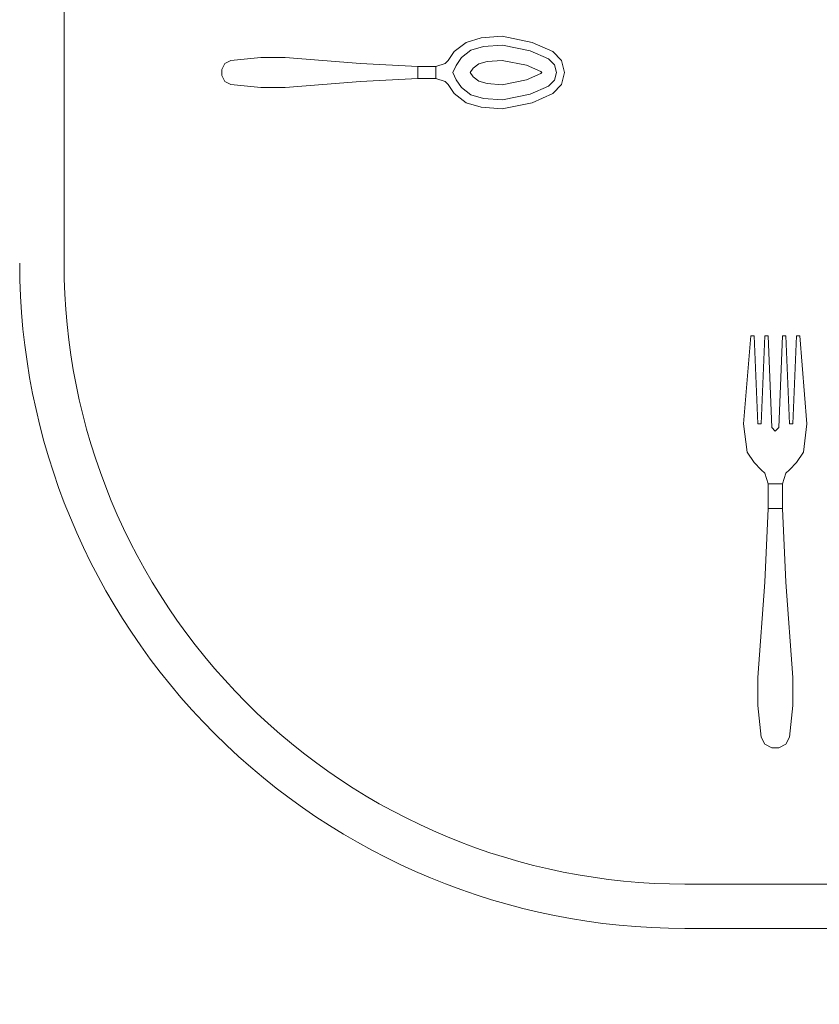
# Model space of a CAD drawing. Units: inches. Extents: x 375 to 1122, y 27 to 1069.
# Tile 9 of 155: x 705.14 to 719.12, y 253.38 to 270.59. Entities that reach past the tile are written whole.
import ezdxf

# ---------------------------------------------------------------- set-up
doc = ezdxf.new("R2010")
doc.units = ezdxf.units.IN
doc.layers.add('A-ANNO-DIMS', color=2, linetype='Continuous', lineweight=18)
doc.layers.add('Furniture', color=30, linetype='Continuous', lineweight=18)
doc.styles.get("Standard").update_dxf_attribs({"font": 'arial.ttf'})
doc.dimstyles.new('ISO-25', dxfattribs={"dimtxt": 12, "dimasz": 2.5, "dimexe": 1.5, "dimexo": 1.5, "dimtad": 1, "dimdec": 1, "dimlunit": 3, "dimtxsty": 'Standard', "dimblk": 'ARCHTICK', "dimcen": 2.5, "dimadec": 0, "dimazin": 0, "dimtfac": 1, "dimtdec": 1, "dimtmove": 0, "dimatfit": 3, "dimfxl": 1.5, "dimfxlon": 1, "dimarcsym": 0})

# ---------------------------------------------------------------- blocks, each defined once
blk = doc.blocks.new('A$C403C54AD')
for p, q in [((2.27071, 1.26108, -0.0006), (2.27071, 0.79569, -0.0006)), ((2.2901, 1.26108, -0.0006), (2.2901, 0.79569, -0.0006)), ((2.08179, 0.82287, -0.05014), (2.08641, 0.82595, -0.04968)), ((2.08179, 0.82287, -0.05322), (2.08641, 0.82595, -0.05276)), ((0.83575, 0.52421, -0.0006), (1.99923, 0.52421, -0.0006))]:
    blk.add_line(p, q)
for radius in [0.27148, 0.29087]:
    blk.add_arc((1.99923, 0.79569, -0.0006), radius, 270, 0)
for points, invisible_edges in [([(2.06948, 0.84288, -0.04954), (2.06948, 0.84903, -0.04954), (2.031, 0.84596, -0.04244), (2.031, 0.84442, -0.04244)], 1), ([(2.06948, 0.84288, -0.05262), (2.06948, 0.84903, -0.05262), (2.031, 0.84596, -0.04552), (2.031, 0.84442, -0.04552)], 1), ([(2.08179, 0.84749, -0.05014), (2.06948, 0.84134, -0.04954), (2.06948, 0.84288, -0.04954), (2.06948, 0.84903, -0.04954)], 5), ([(2.08179, 0.84749, -0.05322), (2.06948, 0.84134, -0.05262), (2.06948, 0.84288, -0.05262), (2.06948, 0.84903, -0.05262)], 5), ([(2.08179, 0.84749, -0.05014), (2.08179, 0.84749, -0.05322), (2.06948, 0.84903, -0.05262), (2.06948, 0.84903, -0.04954)], 1), ([(2.08179, 0.84749, -0.05014), (2.07268, 0.83518, -0.04994), (2.07102, 0.83672, -0.04979), (2.06948, 0.84134, -0.04954)], 13), ([(2.08179, 0.84749, -0.05322), (2.07268, 0.83518, -0.05301), (2.07102, 0.83672, -0.05286), (2.06948, 0.84134, -0.05262)], 13), ([(2.08179, 0.84749, -0.05014), (2.07268, 0.83518, -0.04994), (2.08179, 0.82287, -0.05014), (2.08179, 0.84749, -0.05014)], 7), ([(2.08179, 0.84749, -0.05322), (2.07268, 0.83518, -0.05301), (2.08179, 0.82287, -0.05322), (2.08179, 0.84749, -0.05322)], 7), ([(2.08641, 0.84442, -0.04968), (2.08641, 0.82595, -0.04968), (2.08179, 0.82287, -0.05014), (2.08179, 0.84749, -0.05014)], 5), ([(2.08641, 0.84442, -0.05276), (2.08641, 0.82595, -0.05276), (2.08179, 0.82287, -0.05322), (2.08179, 0.84749, -0.05322)], 5), ([(2.08641, 0.84442, -0.05276), (2.08641, 0.84442, -0.04968), (2.08179, 0.84749, -0.05014), (2.08179, 0.84749, -0.05322)], 4), ([(2.08949, 0.82902, -0.05152), (2.08949, 0.84134, -0.05152), (2.08641, 0.84442, -0.05276), (2.08641, 0.82595, -0.05276)], 5), ([(2.08949, 0.82902, -0.04844), (2.08949, 0.84134, -0.04844), (2.08641, 0.84442, -0.04968), (2.08641, 0.82595, -0.04968)], 5), ([(2.06948, 0.84134, -0.04954), (2.07102, 0.83672, -0.04979), (2.031, 0.83826, -0.04244), (2.031, 0.8398, -0.04244)], 1), ([(2.06948, 0.84134, -0.05262), (2.07102, 0.83672, -0.05286), (2.031, 0.83826, -0.04552), (2.031, 0.8398, -0.04552)], 1), ([(2.09103, 0.83056, -0.04739), (2.09103, 0.8398, -0.04739), (2.08949, 0.84134, -0.04844), (2.08949, 0.82902, -0.04844)], 5), ([(2.09103, 0.83056, -0.05018), (2.09103, 0.8398, -0.05018), (2.08949, 0.84134, -0.05152), (2.08949, 0.82902, -0.05152)], 5), ([(2.09103, 0.8398, -0.05018), (2.09103, 0.8398, -0.04739), (2.08949, 0.84134, -0.04844), (2.08949, 0.84134, -0.05152)], 1), ([(2.09564, 0.83826, -0.04504), (2.09564, 0.8321, -0.04504), (2.09103, 0.83056, -0.04739), (2.09103, 0.8398, -0.04739)], 4), ([(2.09564, 0.83826, -0.04763), (2.09564, 0.8321, -0.04763), (2.09103, 0.83056, -0.05018), (2.09103, 0.8398, -0.05018)], 4), ([(2.09564, 0.83826, -0.04504), (2.09564, 0.83826, -0.04763), (2.09103, 0.8398, -0.05018), (2.09103, 0.8398, -0.04739)], 5), ([(2.13874, 0.8398, -0.04587), (2.13874, 0.83056, -0.04587), (2.10642, 0.8321, -0.04296), (2.10642, 0.83826, -0.04296)], 1), ([(2.13874, 0.8398, -0.04587), (2.13874, 0.8398, -0.04895), (2.10642, 0.83826, -0.04555), (2.10642, 0.83826, -0.04296)], 5), ([(2.13874, 0.8398, -0.04895), (2.13874, 0.83056, -0.04895), (2.10642, 0.8321, -0.04555), (2.10642, 0.83826, -0.04555)], 1), ([(2.1803, 0.82749, -0.04825), (2.1803, 0.84288, -0.04825), (2.13874, 0.8398, -0.04587), (2.13874, 0.83056, -0.04587)], 5), ([(2.1803, 0.82749, -0.05289), (2.1803, 0.84288, -0.05289), (2.13874, 0.8398, -0.04895), (2.13874, 0.83056, -0.04895)], 5), ([(2.1803, 0.84288, -0.05289), (2.1803, 0.84288, -0.04825), (2.13874, 0.8398, -0.04587), (2.13874, 0.8398, -0.04895)], 4), ([(2.19261, 0.84288, -0.04858), (2.19261, 0.82749, -0.04858), (2.1803, 0.82749, -0.04825), (2.1803, 0.84288, -0.04825)], 5), ([(2.19261, 0.84288, -0.05321), (2.19261, 0.82749, -0.05321), (2.1803, 0.82749, -0.05289), (2.1803, 0.84288, -0.05289)], 5), ([(2.20647, 0.82902, -0.04855), (2.20647, 0.84134, -0.04855), (2.19261, 0.84288, -0.04858), (2.19261, 0.82749, -0.04858)], 5), ([(2.20647, 0.82902, -0.05318), (2.20647, 0.84134, -0.05318), (2.19261, 0.84288, -0.05321), (2.19261, 0.82749, -0.05321)], 5), ([(2.20954, 0.8398, -0.0483), (2.20954, 0.83056, -0.0483), (2.20647, 0.82902, -0.04855), (2.20647, 0.84134, -0.04855)], 5), ([(2.20954, 0.8398, -0.05294), (2.20954, 0.83056, -0.05294), (2.20647, 0.82902, -0.05318), (2.20647, 0.84134, -0.05318)], 5), ([(2.21108, 0.83364, -0.04847), (2.21108, 0.83672, -0.04847), (2.20954, 0.8398, -0.0483), (2.20954, 0.83056, -0.0483)], 4), ([(2.21108, 0.83364, -0.0526), (2.21108, 0.83672, -0.0526), (2.20954, 0.8398, -0.05294), (2.20954, 0.83056, -0.05294)], 4), ([(2.10642, 0.83826, -0.04555), (2.10642, 0.83826, -0.04296), (2.09564, 0.83826, -0.04504), (2.09564, 0.83826, -0.04763)], 5), ([(2.07102, 0.83364, -0.04979), (2.06948, 0.82902, -0.04954), (2.031, 0.83056, -0.04244), (2.031, 0.8321, -0.04244)], 1), ([(2.07102, 0.83364, -0.05286), (2.06948, 0.82902, -0.05262), (2.031, 0.83056, -0.04552), (2.031, 0.8321, -0.04552)], 1), ([(2.08179, 0.82287, -0.05014), (2.07268, 0.83518, -0.04994), (2.07102, 0.83364, -0.04979), (2.06948, 0.82902, -0.04954)], 13), ([(2.08179, 0.82287, -0.05322), (2.07268, 0.83518, -0.05301), (2.07102, 0.83364, -0.05286), (2.06948, 0.82902, -0.05262)], 13), ([(2.09564, 0.8321, -0.04763), (2.09564, 0.8321, -0.04504), (2.09103, 0.83056, -0.04739), (2.09103, 0.83056, -0.05018)], 5), ([(2.09564, 0.8321, -0.04763), (2.09564, 0.8321, -0.04504), (2.10642, 0.8321, -0.04296), (2.10642, 0.8321, -0.04555)], 5), ([(2.10642, 0.8321, -0.04296), (2.10642, 0.8321, -0.04555), (2.13874, 0.83056, -0.04895), (2.13874, 0.83056, -0.04587)], 5), ([(2.06948, 0.82749, -0.04954), (2.06948, 0.82133, -0.04954), (2.031, 0.82441, -0.04244), (2.031, 0.82595, -0.04244)], 1), ([(2.06948, 0.82749, -0.05262), (2.06948, 0.82133, -0.05262), (2.031, 0.82441, -0.04552), (2.031, 0.82595, -0.04552)], 1), ([(2.08179, 0.82287, -0.05014), (2.06948, 0.82902, -0.04954), (2.06948, 0.82749, -0.04954), (2.06948, 0.82133, -0.04954)], 5), ([(2.08179, 0.82287, -0.05322), (2.06948, 0.82902, -0.05262), (2.06948, 0.82749, -0.05262), (2.06948, 0.82133, -0.05262)], 5), ([(2.09103, 0.83056, -0.04739), (2.09103, 0.83056, -0.05018), (2.08949, 0.82902, -0.05152), (2.08949, 0.82902, -0.04844)], 1), ([(2.13874, 0.83056, -0.04895), (2.13874, 0.83056, -0.04587), (2.1803, 0.82749, -0.04825), (2.1803, 0.82749, -0.05289)], 1), ([(2.08179, 0.82287, -0.05322), (2.08179, 0.82287, -0.05014), (2.06948, 0.82133, -0.04954), (2.06948, 0.82133, -0.05262)], 1), ([(2.08641, 0.82595, -0.04968), (2.08641, 0.82595, -0.05276), (2.08179, 0.82287, -0.05322), (2.08179, 0.82287, -0.05014)], 4), ([(1.90985, 0.73605, -0.02421), (1.9066, 0.73789, -0.02157), (1.91055, 0.74173, -0.02048), (1.91253, 0.73867, -0.02365)], 5), ([(1.90985, 0.73605, -0.02289), (1.9066, 0.73789, -0.02025), (1.91055, 0.74173, -0.01916), (1.91253, 0.73867, -0.02233)], 5), ([(1.91055, 0.74173, -0.02048), (1.91253, 0.73867, -0.02365), (1.91583, 0.73948, -0.02346), (1.91583, 0.74304, -0.02029)], 5), ([(1.91055, 0.74173, -0.01916), (1.91253, 0.73867, -0.02233), (1.91583, 0.73948, -0.02215), (1.91583, 0.74304, -0.01897)], 5), ([(1.92111, 0.74173, -0.02048), (1.91914, 0.73867, -0.02365), (1.91583, 0.73948, -0.02346), (1.91583, 0.74304, -0.02029)], 5), ([(1.92111, 0.74173, -0.01916), (1.91914, 0.73867, -0.02233), (1.91583, 0.73948, -0.02215), (1.91583, 0.74304, -0.01897)], 5), ([(1.92182, 0.73605, -0.02421), (1.92507, 0.73789, -0.02157), (1.92111, 0.74173, -0.02048), (1.91914, 0.73867, -0.02365)], 5), ([(1.92182, 0.73605, -0.02289), (1.92507, 0.73789, -0.02025), (1.92111, 0.74173, -0.01916), (1.91914, 0.73867, -0.02233)], 5), ([(1.90264, 0.72882, -0.0234), (1.90634, 0.72802, -0.02592), (1.90985, 0.73605, -0.02421), (1.9066, 0.73789, -0.02157)], 5), ([(1.90264, 0.72882, -0.02208), (1.90634, 0.72802, -0.0246), (1.90985, 0.73605, -0.02289), (1.9066, 0.73789, -0.02025)], 5), ([(1.9154, 0.73267, -0.02578), (1.91253, 0.73867, -0.02233), (1.90985, 0.73605, -0.02289), (1.9154, 0.73267, -0.02578)], 5), ([(1.9154, 0.73267, -0.0271), (1.91253, 0.73867, -0.02365), (1.90985, 0.73605, -0.02421), (1.9154, 0.73267, -0.0271)], 5), ([(1.91583, 0.73948, -0.02215), (1.91583, 0.73309, -0.02564), (1.9154, 0.73267, -0.02578), (1.91253, 0.73867, -0.02233)], 5), ([(1.91583, 0.73948, -0.02346), (1.91583, 0.73309, -0.02696), (1.9154, 0.73267, -0.0271), (1.91253, 0.73867, -0.02365)], 5), ([(1.91583, 0.73948, -0.02215), (1.91583, 0.73309, -0.02564), (1.91627, 0.73267, -0.02578), (1.91914, 0.73867, -0.02233)], 5), ([(1.91583, 0.73948, -0.02346), (1.91583, 0.73309, -0.02696), (1.91627, 0.73267, -0.0271), (1.91914, 0.73867, -0.02365)], 5), ([(1.91627, 0.73267, -0.02578), (1.91914, 0.73867, -0.02233), (1.92182, 0.73605, -0.02289), (1.91627, 0.73267, -0.02578)], 5), ([(1.91627, 0.73267, -0.0271), (1.91914, 0.73867, -0.02365), (1.92182, 0.73605, -0.02421), (1.91627, 0.73267, -0.0271)], 5), ([(1.92903, 0.72882, -0.0234), (1.92532, 0.72802, -0.02592), (1.92182, 0.73605, -0.02421), (1.92507, 0.73789, -0.02157)], 5), ([(1.92903, 0.72882, -0.02208), (1.92532, 0.72802, -0.0246), (1.92182, 0.73605, -0.02289), (1.92507, 0.73789, -0.02025)], 5), ([(1.90985, 0.73605, -0.02421), (1.9154, 0.73267, -0.0271), (1.91266, 0.72644, -0.02873), (1.90634, 0.72802, -0.02592)], 5), ([(1.90985, 0.73605, -0.02289), (1.9154, 0.73267, -0.02578), (1.91266, 0.72644, -0.02741), (1.90634, 0.72802, -0.0246)], 5), ([(1.9154, 0.73267, -0.0271), (1.91627, 0.73267, -0.0271), (1.91901, 0.72644, -0.02873), (1.91266, 0.72644, -0.02873)], 5), ([(1.9154, 0.73267, -0.02578), (1.91627, 0.73267, -0.02578), (1.91901, 0.72644, -0.02741), (1.91266, 0.72644, -0.02741)], 5), ([(1.91583, 0.73309, -0.02564), (1.91627, 0.73267, -0.02578), (1.9154, 0.73267, -0.02578), (1.91583, 0.73309, -0.02564)], 2), ([(1.91583, 0.73309, -0.02696), (1.91627, 0.73267, -0.0271), (1.9154, 0.73267, -0.0271), (1.91583, 0.73309, -0.02696)], 2), ([(1.92182, 0.73605, -0.02421), (1.91627, 0.73267, -0.0271), (1.91901, 0.72644, -0.02873), (1.92532, 0.72802, -0.02592)], 5), ([(1.92182, 0.73605, -0.02289), (1.91627, 0.73267, -0.02578), (1.91901, 0.72644, -0.02741), (1.92532, 0.72802, -0.0246)], 5), ([(1.90388, 0.71589, -0.0279), (1.9, 0.71579, -0.02544), (1.90264, 0.72882, -0.0234), (1.90634, 0.72802, -0.02592)], 5), ([(1.90388, 0.71589, -0.02658), (1.9, 0.71579, -0.02412), (1.90264, 0.72882, -0.02208), (1.90634, 0.72802, -0.0246)], 5), ([(1.91266, 0.72644, -0.02741), (1.90634, 0.72802, -0.0246), (1.90388, 0.71589, -0.02658), (1.91051, 0.71583, -0.02912)], 5), ([(1.91266, 0.72644, -0.02873), (1.90634, 0.72802, -0.02592), (1.90388, 0.71589, -0.0279), (1.91051, 0.71583, -0.03044)], 5), ([(1.91901, 0.72644, -0.02741), (1.92532, 0.72802, -0.0246), (1.92778, 0.71589, -0.02658), (1.92116, 0.71583, -0.02912)], 5), ([(1.91901, 0.72644, -0.02873), (1.92532, 0.72802, -0.02592), (1.92778, 0.71589, -0.0279), (1.92116, 0.71583, -0.03044)], 5), ([(1.92778, 0.71589, -0.0279), (1.93166, 0.71579, -0.02544), (1.92903, 0.72882, -0.0234), (1.92532, 0.72802, -0.02592)], 5), ([(1.92778, 0.71589, -0.02658), (1.93166, 0.71579, -0.02412), (1.92903, 0.72882, -0.02208), (1.92532, 0.72802, -0.0246)], 5), ([(1.91901, 0.72644, -0.02741), (1.91266, 0.72644, -0.02741), (1.91051, 0.71583, -0.02912), (1.92116, 0.71583, -0.02912)], 5), ([(1.91901, 0.72644, -0.02873), (1.91266, 0.72644, -0.02873), (1.91051, 0.71583, -0.03044), (1.92116, 0.71583, -0.03044)], 5), ([(1.90066, 0.70658, -0.02499), (1.90447, 0.70765, -0.02747), (1.90388, 0.71589, -0.02658), (1.9, 0.71579, -0.02412)], 5), ([(1.90066, 0.70658, -0.02631), (1.90447, 0.70765, -0.02879), (1.90388, 0.71589, -0.0279), (1.9, 0.71579, -0.02544)], 5), ([(1.90388, 0.71589, -0.0279), (1.91051, 0.71583, -0.03044), (1.91098, 0.70922, -0.03139), (1.90447, 0.70765, -0.02879)], 5), ([(1.90388, 0.71589, -0.02658), (1.91051, 0.71583, -0.02912), (1.91098, 0.70922, -0.03007), (1.90447, 0.70765, -0.02747)], 5), ([(1.91051, 0.71583, -0.03044), (1.92116, 0.71583, -0.03044), (1.92068, 0.70922, -0.03139), (1.91098, 0.70922, -0.03139)], 5), ([(1.91051, 0.71583, -0.02912), (1.92116, 0.71583, -0.02912), (1.92068, 0.70922, -0.03007), (1.91098, 0.70922, -0.03007)], 5), ([(1.92778, 0.71589, -0.0279), (1.92116, 0.71583, -0.03044), (1.92068, 0.70922, -0.03139), (1.92719, 0.70765, -0.02879)], 5), ([(1.92778, 0.71589, -0.02658), (1.92116, 0.71583, -0.02912), (1.92068, 0.70922, -0.03007), (1.92719, 0.70765, -0.02747)], 5), ([(1.931, 0.70658, -0.02499), (1.92719, 0.70765, -0.02747), (1.92778, 0.71589, -0.02658), (1.93166, 0.71579, -0.02412)], 5), ([(1.931, 0.70658, -0.02631), (1.92719, 0.70765, -0.02879), (1.92778, 0.71589, -0.0279), (1.93166, 0.71579, -0.02544)], 5), ([(1.90613, 0.70213, -0.02798), (1.90264, 0.69998, -0.02539), (1.90066, 0.70658, -0.02499), (1.90447, 0.70765, -0.02747)], 5), ([(1.90613, 0.70213, -0.0293), (1.90264, 0.69998, -0.02671), (1.90066, 0.70658, -0.02631), (1.90447, 0.70765, -0.02879)], 5), ([(1.91098, 0.70922, -0.03007), (1.90447, 0.70765, -0.02747), (1.90613, 0.70213, -0.02798), (1.9121, 0.7055, -0.0303)], 5), ([(1.92068, 0.70922, -0.03139), (1.91098, 0.70922, -0.03139), (1.9121, 0.7055, -0.03162), (1.91956, 0.7055, -0.03162)], 5), ([(1.92068, 0.70922, -0.03007), (1.91098, 0.70922, -0.03007), (1.9121, 0.7055, -0.0303), (1.91956, 0.7055, -0.0303)], 5), ([(1.92068, 0.70922, -0.03139), (1.92719, 0.70765, -0.02879), (1.92553, 0.70213, -0.0293), (1.91956, 0.7055, -0.03162)], 5), ([(1.92068, 0.70922, -0.03007), (1.92719, 0.70765, -0.02747), (1.92553, 0.70213, -0.02798), (1.91956, 0.7055, -0.0303)], 5), ([(1.92553, 0.70213, -0.02798), (1.92903, 0.69998, -0.02539), (1.931, 0.70658, -0.02499), (1.92719, 0.70765, -0.02747)], 5), ([(1.92553, 0.70213, -0.0293), (1.92903, 0.69998, -0.02671), (1.931, 0.70658, -0.02631), (1.92719, 0.70765, -0.02879)], 5), ([(1.9066, 0.69472, -0.02719), (1.90928, 0.69791, -0.02947), (1.90613, 0.70213, -0.0293), (1.90264, 0.69998, -0.02671)], 5), ([(1.9066, 0.69472, -0.02588), (1.90928, 0.69791, -0.02815), (1.90613, 0.70213, -0.02798), (1.90264, 0.69998, -0.02539)], 5), ([(1.90613, 0.70213, -0.0293), (1.9121, 0.7055, -0.03162), (1.91387, 0.70313, -0.03172), (1.90928, 0.69791, -0.02947)], 5), ([(1.90613, 0.70213, -0.02798), (1.9121, 0.7055, -0.0303), (1.91387, 0.70313, -0.0304), (1.90928, 0.69791, -0.02815)], 5), ([(1.91387, 0.70313, -0.03172), (1.90928, 0.69791, -0.02947), (1.91269, 0.69562, -0.02948), (1.91583, 0.70178, -0.03152)], 5), ([(1.91387, 0.70313, -0.0304), (1.90928, 0.69791, -0.02815), (1.91269, 0.69562, -0.02816), (1.91583, 0.70178, -0.0302)], 5), ([(1.9121, 0.7055, -0.03162), (1.91956, 0.7055, -0.03162), (1.91779, 0.70313, -0.03172), (1.91387, 0.70313, -0.03172)], 5), ([(1.9121, 0.7055, -0.0303), (1.91956, 0.7055, -0.0303), (1.91779, 0.70313, -0.0304), (1.91387, 0.70313, -0.0304)], 5), ([(1.91269, 0.69562, -0.02948), (1.91583, 0.70178, -0.03152), (1.91583, 0.70178, -0.03152), (1.91583, 0.69426, -0.0293)], 5), ([(1.91269, 0.69562, -0.02816), (1.91583, 0.70178, -0.0302), (1.91583, 0.70178, -0.0302), (1.91583, 0.69426, -0.02798)], 5), ([(1.91779, 0.70313, -0.03172), (1.91387, 0.70313, -0.03172), (1.91583, 0.70178, -0.03152)], 1), ([(1.91779, 0.70313, -0.0304), (1.91387, 0.70313, -0.0304), (1.91583, 0.70178, -0.0302)], 1), ([(1.91779, 0.70313, -0.03172), (1.92238, 0.69791, -0.02947), (1.91897, 0.69562, -0.02948), (1.91583, 0.70178, -0.03152)], 5), ([(1.91779, 0.70313, -0.0304), (1.92238, 0.69791, -0.02815), (1.91897, 0.69562, -0.02816), (1.91583, 0.70178, -0.0302)], 5), ([(1.91897, 0.69562, -0.02948), (1.91583, 0.70178, -0.03152), (1.91583, 0.70178, -0.03152), (1.91583, 0.69426, -0.0293)], 5), ([(1.91897, 0.69562, -0.02816), (1.91583, 0.70178, -0.0302), (1.91583, 0.70178, -0.0302), (1.91583, 0.69426, -0.02798)], 5), ([(1.92553, 0.70213, -0.0293), (1.91956, 0.7055, -0.03162), (1.91779, 0.70313, -0.03172), (1.92238, 0.69791, -0.02947)], 5), ([(1.92553, 0.70213, -0.02798), (1.91956, 0.7055, -0.0303), (1.91779, 0.70313, -0.0304), (1.92238, 0.69791, -0.02815)], 5), ([(1.92507, 0.69472, -0.02719), (1.92238, 0.69791, -0.02947), (1.92553, 0.70213, -0.0293), (1.92903, 0.69998, -0.02671)], 5), ([(1.92507, 0.69472, -0.02588), (1.92238, 0.69791, -0.02815), (1.92553, 0.70213, -0.02798), (1.92903, 0.69998, -0.02539)], 5), ([(1.91269, 0.69562, -0.02816), (1.91055, 0.6921, -0.02625), (1.9066, 0.69472, -0.02588), (1.90928, 0.69791, -0.02815)], 5), ([(1.91897, 0.69562, -0.02948), (1.92111, 0.6921, -0.0284), (1.92507, 0.69472, -0.02719), (1.92238, 0.69791, -0.02947)], 5), ([(1.91897, 0.69562, -0.02816), (1.92111, 0.6921, -0.02625), (1.92507, 0.69472, -0.02588), (1.92238, 0.69791, -0.02815)], 5), ([(1.91055, 0.6921, -0.0284), (1.91583, 0.6921, -0.0284), (1.91583, 0.69426, -0.0293), (1.91269, 0.69562, -0.02948)], 11), ([(1.91055, 0.6921, -0.02625), (1.91583, 0.6921, -0.02625), (1.91583, 0.69426, -0.02798), (1.91269, 0.69562, -0.02816)], 11), ([(1.92111, 0.6921, -0.0284), (1.91583, 0.6921, -0.0284), (1.91583, 0.69426, -0.0293), (1.91897, 0.69562, -0.02948)], 11), ([(1.92111, 0.6921, -0.02625), (1.91583, 0.6921, -0.02625), (1.91583, 0.69426, -0.02798), (1.91897, 0.69562, -0.02816)], 11), ([(1.91187, 0.69077, -0.02551), (1.91979, 0.69077, -0.02551), (1.92111, 0.6921, -0.02625), (1.91055, 0.6921, -0.02625)], 5), ([(1.91187, 0.69077, -0.0276), (1.91979, 0.69077, -0.0276), (1.92111, 0.6921, -0.0284), (1.91055, 0.6921, -0.0284)], 5), ([(1.91187, 0.69077, -0.02551), (1.91187, 0.69077, -0.0276), (1.91055, 0.6921, -0.0284), (1.91055, 0.6921, -0.02625)], 1), ([(1.91847, 0.68681, -0.02366), (1.91319, 0.68681, -0.02366), (1.91187, 0.69077, -0.02551), (1.91979, 0.69077, -0.02551)], 4), ([(1.91319, 0.68681, -0.02588), (1.91319, 0.68681, -0.02366), (1.91187, 0.69077, -0.02551), (1.91187, 0.69077, -0.0276)], 5), ([(1.91847, 0.68681, -0.02588), (1.91319, 0.68681, -0.02588), (1.91187, 0.69077, -0.0276), (1.91979, 0.69077, -0.0276)], 4), ([(1.91847, 0.68681, -0.02366), (1.91847, 0.68681, -0.02588), (1.91979, 0.69077, -0.0276), (1.91979, 0.69077, -0.02551)], 5), ([(1.91979, 0.69077, -0.0276), (1.91979, 0.69077, -0.02551), (1.92111, 0.6921, -0.02625), (1.92111, 0.6921, -0.0284)], 1), ([(1.91319, 0.68681, -0.02588), (1.91319, 0.68681, -0.02366), (1.91319, 0.6789, -0.02303), (1.91319, 0.6789, -0.02525)], 5), ([(1.91847, 0.6789, -0.02525), (1.91847, 0.6789, -0.02303), (1.91847, 0.68681, -0.02366), (1.91847, 0.68681, -0.02588)], 5), ([(1.91979, 0.65383, -0.02553), (1.91187, 0.65383, -0.02553), (1.91319, 0.6789, -0.02303), (1.91847, 0.6789, -0.02303)], 1), ([(1.91319, 0.6789, -0.02303), (1.91319, 0.6789, -0.02525), (1.91187, 0.65383, -0.02816), (1.91187, 0.65383, -0.02553)], 5), ([(1.91979, 0.65383, -0.02816), (1.91187, 0.65383, -0.02816), (1.91319, 0.6789, -0.02525), (1.91847, 0.6789, -0.02525)], 1), ([(1.91979, 0.65383, -0.02553), (1.91979, 0.65383, -0.02816), (1.91847, 0.6789, -0.02525), (1.91847, 0.6789, -0.02303)], 5), ([(1.90924, 0.62085, -0.03154), (1.92243, 0.62085, -0.03154), (1.91979, 0.65383, -0.02816), (1.91187, 0.65383, -0.02816)], 5), ([(1.91187, 0.65383, -0.02816), (1.91187, 0.65383, -0.02553), (1.90924, 0.62085, -0.02757), (1.90924, 0.62085, -0.03154)], 1), ([(1.90924, 0.62085, -0.02757), (1.92243, 0.62085, -0.02757), (1.91979, 0.65383, -0.02553), (1.91187, 0.65383, -0.02553)], 5), ([(1.92243, 0.62085, -0.03154), (1.92243, 0.62085, -0.02757), (1.91979, 0.65383, -0.02553), (1.91979, 0.65383, -0.02816)], 4), ([(1.92243, 0.61029, -0.02785), (1.90924, 0.61029, -0.02785), (1.90924, 0.62085, -0.02757), (1.92243, 0.62085, -0.02757)], 5), ([(1.92243, 0.61029, -0.03182), (1.90924, 0.61029, -0.03182), (1.90924, 0.62085, -0.03154), (1.92243, 0.62085, -0.03154)], 5), ([(1.91055, 0.5971, -0.02782), (1.92111, 0.5971, -0.02782), (1.92243, 0.61029, -0.02785), (1.90924, 0.61029, -0.02785)], 5), ([(1.91055, 0.5971, -0.03179), (1.92111, 0.5971, -0.03179), (1.92243, 0.61029, -0.03182), (1.90924, 0.61029, -0.03182)], 5), ([(1.91979, 0.59446, -0.02761), (1.91187, 0.59446, -0.02761), (1.91055, 0.5971, -0.02782), (1.92111, 0.5971, -0.02782)], 5), ([(1.91979, 0.59446, -0.03158), (1.91187, 0.59446, -0.03158), (1.91055, 0.5971, -0.03179), (1.92111, 0.5971, -0.03179)], 5), ([(1.91451, 0.59314, -0.02775), (1.91715, 0.59314, -0.02775), (1.91979, 0.59446, -0.02761), (1.91187, 0.59446, -0.02761)], 4), ([(1.91451, 0.59314, -0.0313), (1.91715, 0.59314, -0.0313), (1.91979, 0.59446, -0.03158), (1.91187, 0.59446, -0.03158)], 4)]:
    blk.add_3dface(points, dxfattribs=dict(invisible_edges=invisible_edges))
for points in [[(2.06948, 0.84903, -0.05262), (2.06948, 0.84903, -0.04954), (2.031, 0.84596, -0.04244), (2.031, 0.84596, -0.04552)], [(2.031, 0.84596, -0.04552), (2.031, 0.84596, -0.04244), (2.031, 0.84442, -0.04244), (2.031, 0.84442, -0.04552)], [(2.031, 0.84442, -0.04244), (2.031, 0.84442, -0.04552), (2.06948, 0.84288, -0.05262), (2.06948, 0.84288, -0.04954)], [(2.08949, 0.84134, -0.04844), (2.08949, 0.84134, -0.05152), (2.08641, 0.84442, -0.05276), (2.08641, 0.84442, -0.04968)], [(2.06948, 0.84134, -0.05262), (2.06948, 0.84134, -0.04954), (2.031, 0.8398, -0.04244), (2.031, 0.8398, -0.04552)], [(2.031, 0.8398, -0.04552), (2.031, 0.8398, -0.04244), (2.031, 0.83826, -0.04244), (2.031, 0.83826, -0.04552)], [(2.06948, 0.84134, -0.05262), (2.06948, 0.84134, -0.04954), (2.06948, 0.84288, -0.04954), (2.06948, 0.84288, -0.05262)], [(2.19261, 0.84288, -0.04858), (2.19261, 0.84288, -0.05321), (2.1803, 0.84288, -0.05289), (2.1803, 0.84288, -0.04825)], [(2.20647, 0.84134, -0.05318), (2.20647, 0.84134, -0.04855), (2.19261, 0.84288, -0.04858), (2.19261, 0.84288, -0.05321)], [(2.20954, 0.8398, -0.0483), (2.20954, 0.8398, -0.05294), (2.20647, 0.84134, -0.05318), (2.20647, 0.84134, -0.04855)], [(2.21108, 0.83672, -0.0526), (2.21108, 0.83672, -0.04847), (2.20954, 0.8398, -0.0483), (2.20954, 0.8398, -0.05294)], [(2.031, 0.83826, -0.04552), (2.031, 0.83826, -0.04244), (2.07102, 0.83672, -0.04979), (2.07102, 0.83672, -0.05286)], [(2.07268, 0.83518, -0.05301), (2.07268, 0.83518, -0.04994), (2.07102, 0.83672, -0.04979), (2.07102, 0.83672, -0.05286)], [(2.10642, 0.8321, -0.04296), (2.10642, 0.83826, -0.04296), (2.09564, 0.83826, -0.04504), (2.09564, 0.8321, -0.04504)], [(2.10642, 0.8321, -0.04555), (2.10642, 0.83826, -0.04555), (2.09564, 0.83826, -0.04763), (2.09564, 0.8321, -0.04763)], [(2.21108, 0.83364, -0.04847), (2.21108, 0.83364, -0.0526), (2.21108, 0.83672, -0.0526), (2.21108, 0.83672, -0.04847)], [(2.07102, 0.83364, -0.05286), (2.07102, 0.83364, -0.04979), (2.031, 0.8321, -0.04244), (2.031, 0.8321, -0.04552)], [(2.031, 0.8321, -0.04552), (2.031, 0.8321, -0.04244), (2.031, 0.83056, -0.04244), (2.031, 0.83056, -0.04552)], [(2.07102, 0.83364, -0.04979), (2.07102, 0.83364, -0.05286), (2.07268, 0.83518, -0.05301), (2.07268, 0.83518, -0.04994)], [(2.20954, 0.83056, -0.05294), (2.20954, 0.83056, -0.0483), (2.21108, 0.83364, -0.04847), (2.21108, 0.83364, -0.0526)], [(2.031, 0.83056, -0.04244), (2.031, 0.83056, -0.04552), (2.06948, 0.82902, -0.05262), (2.06948, 0.82902, -0.04954)], [(2.06948, 0.82749, -0.04954), (2.06948, 0.82749, -0.05262), (2.031, 0.82595, -0.04552), (2.031, 0.82595, -0.04244)], [(2.06948, 0.82749, -0.04954), (2.06948, 0.82749, -0.05262), (2.06948, 0.82902, -0.05262), (2.06948, 0.82902, -0.04954)], [(2.08949, 0.82902, -0.05152), (2.08949, 0.82902, -0.04844), (2.08641, 0.82595, -0.04968), (2.08641, 0.82595, -0.05276)], [(2.1803, 0.82749, -0.04825), (2.1803, 0.82749, -0.05289), (2.19261, 0.82749, -0.05321), (2.19261, 0.82749, -0.04858)], [(2.19261, 0.82749, -0.05321), (2.19261, 0.82749, -0.04858), (2.20647, 0.82902, -0.04855), (2.20647, 0.82902, -0.05318)], [(2.20647, 0.82902, -0.04855), (2.20647, 0.82902, -0.05318), (2.20954, 0.83056, -0.05294), (2.20954, 0.83056, -0.0483)], [(2.031, 0.82595, -0.04552), (2.031, 0.82595, -0.04244), (2.031, 0.82441, -0.04244), (2.031, 0.82441, -0.04552)], [(2.031, 0.82441, -0.04244), (2.031, 0.82441, -0.04552), (2.06948, 0.82133, -0.05262), (2.06948, 0.82133, -0.04954)], [(1.91055, 0.74173, -0.01916), (1.91055, 0.74173, -0.02048), (1.9066, 0.73789, -0.02157), (1.9066, 0.73789, -0.02025)], [(1.91583, 0.74304, -0.02029), (1.91583, 0.74304, -0.01897), (1.91055, 0.74173, -0.01916), (1.91055, 0.74173, -0.02048)], [(1.92111, 0.74173, -0.01916), (1.92111, 0.74173, -0.02048), (1.91583, 0.74304, -0.02029), (1.91583, 0.74304, -0.01897)], [(1.92507, 0.73789, -0.02157), (1.92507, 0.73789, -0.02025), (1.92111, 0.74173, -0.01916), (1.92111, 0.74173, -0.02048)], [(1.9066, 0.73789, -0.02157), (1.9066, 0.73789, -0.02025), (1.90264, 0.72882, -0.02208), (1.90264, 0.72882, -0.0234)], [(1.92903, 0.72882, -0.02208), (1.92903, 0.72882, -0.0234), (1.92507, 0.73789, -0.02157), (1.92507, 0.73789, -0.02025)], [(1.90264, 0.72882, -0.02208), (1.90264, 0.72882, -0.0234), (1.9, 0.71579, -0.02544), (1.9, 0.71579, -0.02412)], [(1.93166, 0.71579, -0.02544), (1.93166, 0.71579, -0.02412), (1.92903, 0.72882, -0.02208), (1.92903, 0.72882, -0.0234)], [(1.9, 0.71579, -0.02544), (1.9, 0.71579, -0.02412), (1.90066, 0.70658, -0.02499), (1.90066, 0.70658, -0.02631)], [(1.931, 0.70658, -0.02499), (1.931, 0.70658, -0.02631), (1.93166, 0.71579, -0.02544), (1.93166, 0.71579, -0.02412)], [(1.90066, 0.70658, -0.02631), (1.90066, 0.70658, -0.02499), (1.90264, 0.69998, -0.02539), (1.90264, 0.69998, -0.02671)], [(1.92903, 0.69998, -0.02671), (1.92903, 0.69998, -0.02539), (1.931, 0.70658, -0.02499), (1.931, 0.70658, -0.02631)], [(1.90264, 0.69998, -0.02539), (1.90264, 0.69998, -0.02671), (1.9066, 0.69472, -0.02719), (1.9066, 0.69472, -0.02588)], [(1.92507, 0.69472, -0.02588), (1.92507, 0.69472, -0.02719), (1.92903, 0.69998, -0.02671), (1.92903, 0.69998, -0.02539)], [(1.9066, 0.69472, -0.02719), (1.9066, 0.69472, -0.02588), (1.91055, 0.6921, -0.02625), (1.91055, 0.6921, -0.0284)], [(1.92111, 0.6921, -0.0284), (1.92111, 0.6921, -0.02625), (1.92507, 0.69472, -0.02588), (1.92507, 0.69472, -0.02719)], [(1.91319, 0.6789, -0.02525), (1.91847, 0.6789, -0.02525), (1.91847, 0.68681, -0.02588), (1.91319, 0.68681, -0.02588)], [(1.91319, 0.6789, -0.02303), (1.91847, 0.6789, -0.02303), (1.91847, 0.68681, -0.02366), (1.91319, 0.68681, -0.02366)], [(1.90924, 0.62085, -0.02757), (1.90924, 0.62085, -0.03154), (1.90924, 0.61029, -0.03182), (1.90924, 0.61029, -0.02785)], [(1.92243, 0.61029, -0.02785), (1.92243, 0.61029, -0.03182), (1.92243, 0.62085, -0.03154), (1.92243, 0.62085, -0.02757)], [(1.90924, 0.61029, -0.03182), (1.90924, 0.61029, -0.02785), (1.91055, 0.5971, -0.02782), (1.91055, 0.5971, -0.03179)], [(1.92111, 0.5971, -0.03179), (1.92111, 0.5971, -0.02782), (1.92243, 0.61029, -0.02785), (1.92243, 0.61029, -0.03182)], [(1.91055, 0.5971, -0.02782), (1.91055, 0.5971, -0.03179), (1.91187, 0.59446, -0.03158), (1.91187, 0.59446, -0.02761)], [(1.91187, 0.59446, -0.03158), (1.91187, 0.59446, -0.02761), (1.91451, 0.59314, -0.02775), (1.91451, 0.59314, -0.0313)], [(1.91715, 0.59314, -0.0313), (1.91715, 0.59314, -0.02775), (1.91979, 0.59446, -0.02761), (1.91979, 0.59446, -0.03158)], [(1.91979, 0.59446, -0.02761), (1.91979, 0.59446, -0.03158), (1.92111, 0.5971, -0.03179), (1.92111, 0.5971, -0.02782)], [(1.91451, 0.59314, -0.02775), (1.91451, 0.59314, -0.0313), (1.91715, 0.59314, -0.0313), (1.91715, 0.59314, -0.02775)]]:
    blk.add_3dface(points)
blk = doc.blocks.new('_ArchTick')
at = {"color": 0, "linetype": 'ByBlock', "const_width": 0.15}
blk.add_lwpolyline([(-0.5, -0.5), (0.5, 0.5)], dxfattribs=at)
blk = doc.blocks.new('*D59')
at = {"layer": 'A-ANNO-DIMS', "color": 0, "lineweight": -2, "transparency": 16777216}
for p, q in [((668.717, 346.851), (665.717, 346.851)), ((667.217, 346.851), (667.217, 232.348)), ((668.717, 232.348), (665.717, 232.348)), ((667.217, 232.348), (667.217, 27.496))]:
    blk.add_line(p, q, dxfattribs=at)
at = {"layer": 'Defpoints', "color": 0, "transparency": 16777216}
for p in [(684.392, 346.851), (667.217, 232.348), (684.392, 232.348)]:
    blk.add_point(p, dxfattribs=at)
at = {"layer": 'A-ANNO-DIMS', "color": 0, "lineweight": -2, "transparency": 16777216, "xscale": 2.5, "yscale": 2.5, "zscale": 2.5}
for p, rotation in [((667.217, 346.851), 90), ((667.217, 232.348), 270)]:
    blk.add_blockref('_ArchTick', p, dxfattribs=dict(at, rotation=rotation))
at = {"layer": 'A-ANNO-DIMS', "color": 0, "transparency": 16777216, "insert": (660.387, 128.672), "char_height": 12, "attachment_point": 5, "rotation": 90}
blk.add_mtext('DINING SET 9\'-6 1/2" TYP.', dxfattribs=at)

msp = doc.modelspace()

# ---------------------------------------------------------------- block references
at = {"layer": 'Furniture', "xscale": 39.9918517141215, "yscale": 39.9918517141215, "zscale": 39.9918517141215, "rotation": 270}
msp.add_blockref('A$C403C54AD', (684.955, 346.287, 0.024), dxfattribs=at)

# ---------------------------------------------------------------- dimensions: what is measured, and where the dimension line sits
at = {"layer": 'A-ANNO-DIMS'}
dim = msp.add_linear_dim(base=(667.217, 232.348), p1=(684.392, 346.851), p2=(684.392, 232.348), angle=270, text='DINING SET <> TYP.', dimstyle='ISO-25', override={"dimdec": 1, "dimlfac": 1, "dimrnd": 0, "dimzin": 1, "dimdsep": 46, "dimlunit": 4, "dimfrac": 2}, dxfattribs=at)
dim.commit()
dim.dimension.update_dxf_attribs({"geometry": '*D59', "text_midpoint": (660.387, 128.672)})

doc.saveas('drawing.dxf')
